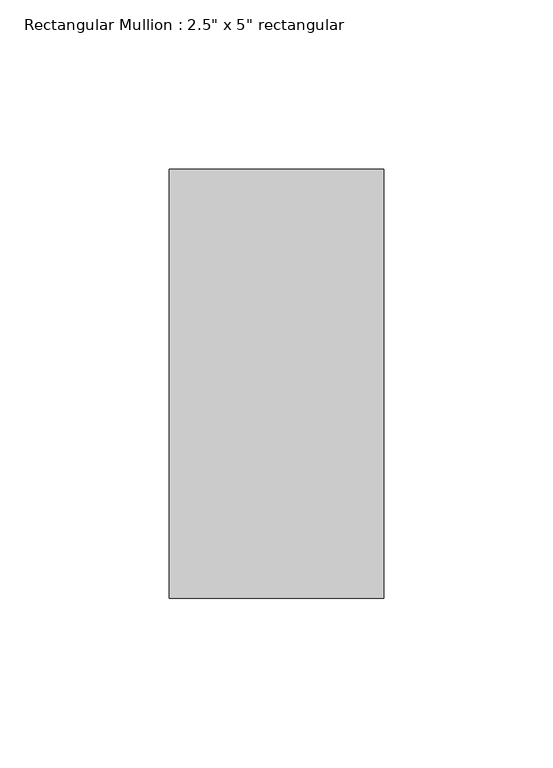
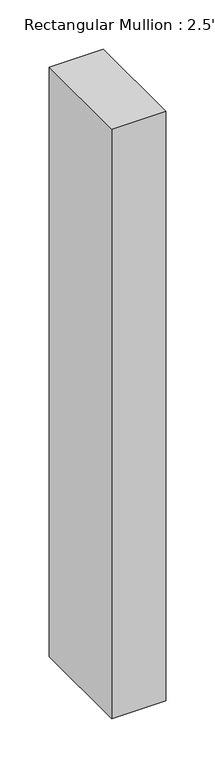
"""IFC4 building model written with IfcOpenShell, lengths in millimetres: member geometry."""

from ifc_helpers import new_model, si_unit, frame, origin, place, context, project, spatial, polyline, outline, extrude, source, transform, mapped, element, save


def member_a689c7fc(model_context):
    return source(origin(), model_context, "Body", "SweptSolid", [
        extrude(outline(polyline([(0.0, 63.5), (0.0, -63.5), (-63.5, -63.5), (-63.5, 63.5), (0.0, 63.5)])), frame((0.0, 0.0, -732.3666667), z_axis=(0.0, 0.0, 1.0), x_axis=(1.0, 0.0, 0.0)), (0.0, 0.0, 1.0), 732.3666667),
    ])


if __name__ == "__main__":
    model = new_model("IFC4")
    model_context = context("Model", 3, world=origin())
    ifc_project = project(units=[si_unit("LENGTHUNIT", "METRE", prefix="MILLI")], contexts=[model_context])
    site = spatial("IfcSite", under=ifc_project)
    building = spatial("IfcBuilding", under=site)
    placement = place(None, origin())
    member_shape = member_a689c7fc(model_context)
    element("IfcMember", 1, ObjectType="Rectangular Mullion : 2.5\" x 5\" rectangular", at=placement, inside=building, context=model_context, shape_type="MappedRepresentation", body=[
        mapped(member_shape, transform((0.0, 0.0, 0.0), x_axis=(1.0, 0.0, 0.0), y_axis=(0.0, 1.0, 0.0), z_axis=(0.0, 0.0, 1.0))),
    ])
    save(model, "model.ifc")

# Revit data of these elements
# Type "Rectangular Mullion : 2.5\" x 5\" rectangular"
#   built-in parameter 1007304 = 0.416667 (stored number, unit not read)
#   built-in parameter 1007301 = 0.104167 (stored number, unit not read)
#   built-in parameter 1007300 = 0.104167 (stored number, unit not read)
# Element 1 (IfcMember, "Rectangular Mullion : 2.5\" x 5\" rectangular")
#   Materials on its faces: "Aluminum"
# Materials
#   "Aluminum": class "Metal", colour RGB 247 247 247, transparency 0, Description = "Aluminum 6061", Cost = 0
